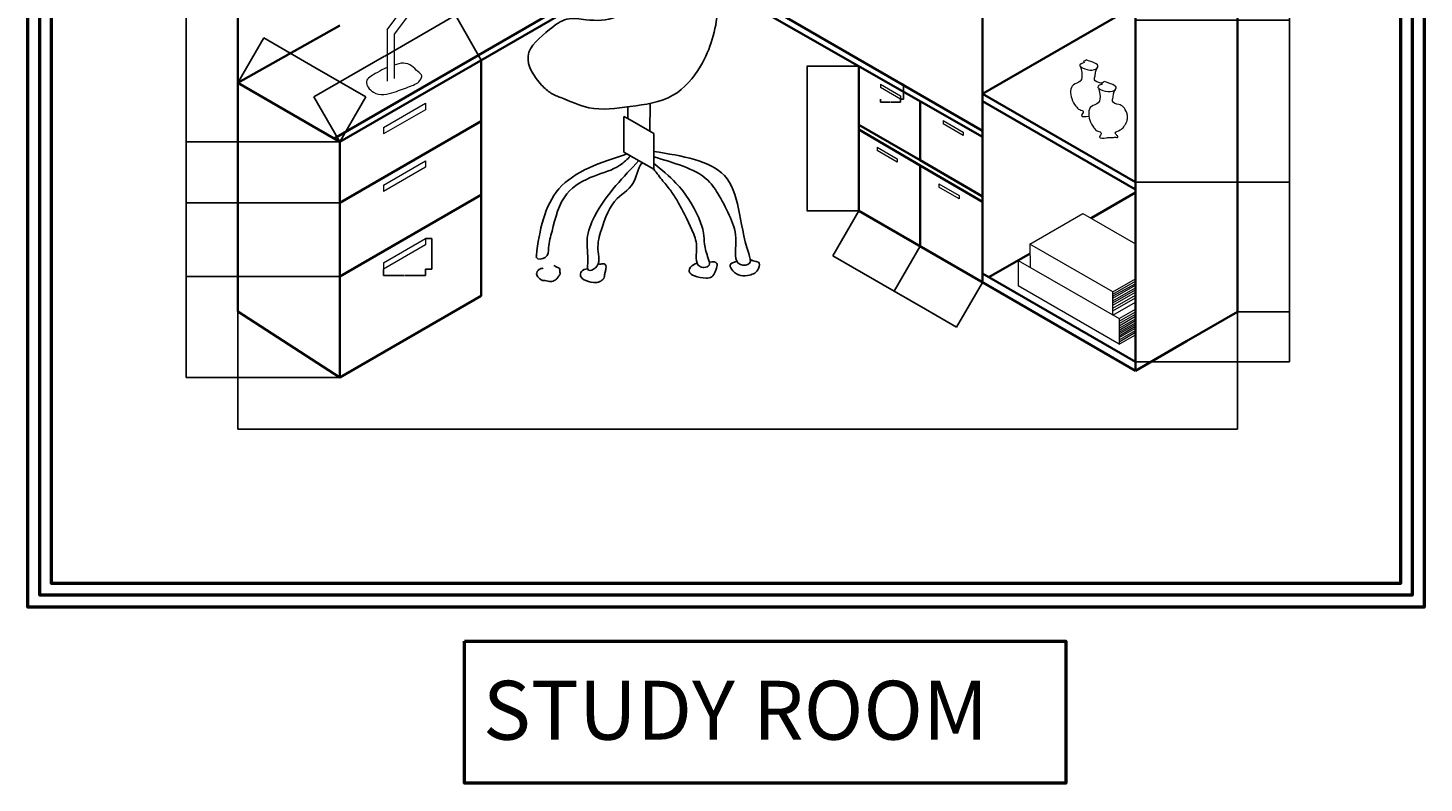
# Model space of a CAD drawing. Units: millimetres. Extents: x -2976 to 8877, y -7187 to 5690.
# Tile 1 of 2: x -2976 to 8877, y -7187 to -776. Entities that reach past the tile are written whole.
import ezdxf

# ---------------------------------------------------------------- set-up
doc = ezdxf.new("R2010")
doc.units = ezdxf.units.MM
doc.header["$MEASUREMENT"] = 0
for name, color, linetype, lineweight in [('A-ANNO-DIMS', 2, 'Continuous', 18), ('A-ANNO-TEXT', 7, 'Continuous', 25), ('A-ANNO-TTLB', 7, 'Continuous', 50), ('A-FURN', 7, 'Continuous', 35), ('A-FURN-ACCS', 3, 'Continuous', 18), ('A-FURN-CHAIR', 4, 'Continuous', 25), ('A-FURN-HDWR', 8, 'Continuous', 18)]:
    doc.layers.add(name, color=color, linetype=linetype, lineweight=lineweight)
doc.styles.get("Standard").update_dxf_attribs({"font": 'arial.ttf'})
doc.dimstyles.get("Standard").update_dxf_attribs({"dimtxt": 0.18, "dimasz": 0.18, "dimexe": 0.18, "dimexo": 0.0625, "dimgap": 0.09, "dimtad": 0, "dimtih": 1, "dimtoh": 1, "dimdec": 0, "dimzin": 0, "dimdsep": 46, "dimtxsty": 'Standard', "dimcen": 0.09, "dimadec": 0, "dimazin": 0, "dimtfac": 1, "dimtdec": 0, "dimtofl": 0, "dimtmove": 0, "dimatfit": 3, "dimfxl": 1, "dimtolj": 1, "dimtzin": 0, "dimarcsym": 0})

# ---------------------------------------------------------------- blocks, each defined once
blk = doc.blocks.new('HANDLE-DRAWER-SMALL')
for p, q in [((0.0001567628432895, 127.2617230564292), (171.3484414772911, 28.33374475136225)), ((0.0001567628432895, 127.2617230564292), (0.0001567628432895, 98.92782070625071)), ((171.3484414772911, -0.0001575988162585), (0.0001567628432895, 98.92782070625049)), ((171.3484414772911, 28.33374475136225), (171.3484414772911, -0.0001575988162585))]:
    blk.add_line(p, q)
blk = doc.blocks.new('HANDLE-DRAWER-LARGE')
for p, q in [((-0.0002251850147701, 53.86751840886313), (355.8206058050919, 259.3007709642777)), ((355.820605805092, 259.3007709642777), (355.820605805092, 205.4328967889142)), ((355.820605805092, 205.4328967889142), (-0.000225185014763, -0.0003557665004337)), ((-0.0002251850147701, 53.86751840886313), (-0.0002251850147701, -0.0003557665004337))]:
    blk.add_line(p, q)
blk = doc.blocks.new('*D5')
at = {"layer": 'A-ANNO-DIMS', "color": 0, "lineweight": -2, "transparency": 16777216}
for p, q in [((4261.184156762843, -1380.200657598816), (4261.184156762843, -1406.020400305983)), ((4261.364156762843, -1405.840400305983), (4344.674786159631, -1405.840400305983)), ((4432.352441477291, -1405.840400305983), (4349.041812080504, -1405.840400305983)), ((4432.532441477291, -1380.200657598816), (4432.532441477291, -1406.020400305983))]:
    blk.add_line(p, q, dxfattribs=at)
at = {"layer": 'A-ANNO-DIMS', "color": 0, "transparency": 16777216}
for points in [[(4261.364156762843, -1405.810400305983), (4261.364156762843, -1405.870400305983), (4261.184156762843, -1405.840400305983)], [(4432.352441477291, -1405.810400305983), (4432.352441477291, -1405.870400305983), (4432.532441477291, -1405.840400305983)]]:
    blk.add_solid(points, dxfattribs=at)
at = {"layer": 'Defpoints', "color": 0, "transparency": 16777216}
for p in [(4261.184156762843, -1380.138157598816), (4432.532441477291, -1380.138157598816), (4432.532441477291, -1405.840400305983)]:
    blk.add_point(p, dxfattribs=at)
at = {"layer": 'A-ANNO-DIMS', "color": 0, "transparency": 16777216, "insert": (4346.858299120067, -1405.840400305983), "char_height": 0.18, "attachment_point": 5}
blk.add_mtext('\\A1;SMALL DRAWER HANDLE 171 TYP.', dxfattribs=at)
blk = doc.blocks.new('*D6')
at = {"layer": 'A-ANNO-DIMS', "color": 0, "lineweight": -2, "transparency": 16777216}
for p, q in [((4432.594941477293, -1252.876276943571), (4458.414684184462, -1252.876276943571)), ((4458.234684184462, -1253.056276943571), (4458.234684184462, -1316.326787530402)), ((4432.594941477293, -1380.138157598816), (4458.414684184462, -1380.138157598816)), ((4458.234684184462, -1379.958157598816), (4458.234684184462, -1316.687647011985))]:
    blk.add_line(p, q, dxfattribs=at)
at = {"layer": 'A-ANNO-DIMS', "color": 0, "transparency": 16777216}
for points in [[(4458.204684184462, -1253.056276943571), (4458.264684184461, -1253.056276943571), (4458.234684184462, -1252.876276943571)], [(4458.204684184462, -1379.958157598816), (4458.264684184461, -1379.958157598816), (4458.234684184462, -1380.138157598816)]]:
    blk.add_solid(points, dxfattribs=at)
at = {"layer": 'Defpoints', "color": 0, "transparency": 16777216}
for p in [(4432.532441477293, -1252.876276943571), (4458.234684184462, -1252.876276943571), (4432.532441477293, -1380.138157598816)]:
    blk.add_point(p, dxfattribs=at)
at = {"layer": 'A-ANNO-DIMS', "color": 0, "transparency": 16777216, "insert": (4458.234684184461, -1316.507217271195), "char_height": 0.18, "attachment_point": 5}
blk.add_mtext('\\A1;127 TYP.', dxfattribs=at)
blk = doc.blocks.new('*D7')
at = {"layer": 'A-ANNO-DIMS', "color": 0, "lineweight": -2, "transparency": 16777216}
for p, q in [((42.54377481498502, -2823.755194985225), (42.54377481498502, -2877.245819633741)), ((398.3646058050918, -2823.755194985225), (398.3646058050918, -2877.245819633741)), ((42.72377481498502, -2877.06581963374), (218.2603021790698, -2877.06581963374)), ((398.1846058050918, -2877.06581963374), (222.648078441007, -2877.06581963374))]:
    blk.add_line(p, q, dxfattribs=at)
at = {"layer": 'A-ANNO-DIMS', "color": 0, "transparency": 16777216}
for points in [[(42.72377481498502, -2877.03581963374), (42.72377481498502, -2877.095819633741), (42.54377481498502, -2877.06581963374)], [(398.1846058050918, -2877.03581963374), (398.1846058050918, -2877.095819633741), (398.3646058050918, -2877.06581963374)]]:
    blk.add_solid(points, dxfattribs=at)
at = {"layer": 'Defpoints', "color": 0, "transparency": 16777216}
for p in [(42.54377481498502, -2823.692694985225), (398.3646058050918, -2823.692694985225), (398.3646058050918, -2877.06581963374)]:
    blk.add_point(p, dxfattribs=at)
at = {"layer": 'A-ANNO-DIMS', "color": 0, "transparency": 16777216, "insert": (220.4541903100384, -2877.06581963374), "char_height": 0.18, "attachment_point": 5}
blk.add_mtext('\\A1;LARGE DRAWER HANDLE 356 TYP.', dxfattribs=at)
blk = doc.blocks.new('*D8')
at = {"layer": 'A-ANNO-DIMS', "color": 0, "lineweight": -2, "transparency": 16777216}
for p, q in [((398.427105805092, -2564.391568254448), (451.9177304536082, -2564.391568254448)), ((451.7377304536082, -2564.571568254447), (451.7377304536082, -2693.860228482047)), ((451.7377304536082, -2823.512694985226), (451.7377304536082, -2694.224034757627)), ((398.427105805092, -2823.692694985226), (451.9177304536082, -2823.692694985226))]:
    blk.add_line(p, q, dxfattribs=at)
at = {"layer": 'A-ANNO-DIMS', "color": 0, "transparency": 16777216}
for points in [[(451.7077304536082, -2564.571568254447), (451.7677304536081, -2564.571568254447), (451.7377304536082, -2564.391568254448)], [(451.7077304536083, -2823.512694985226), (451.7677304536082, -2823.512694985226), (451.7377304536082, -2823.692694985226)]]:
    blk.add_solid(points, dxfattribs=at)
at = {"layer": 'Defpoints', "color": 0, "transparency": 16777216}
for p in [(398.364605805092, -2564.391568254448), (451.7377304536082, -2564.391568254448), (398.364605805092, -2823.692694985226)]:
    blk.add_point(p, dxfattribs=at)
at = {"layer": 'A-ANNO-DIMS', "color": 0, "transparency": 16777216, "insert": (451.7377304536073, -2694.042131619836), "char_height": 0.18, "attachment_point": 5}
blk.add_mtext('\\A1;259 TYP.', dxfattribs=at)
blk = doc.blocks.new('*D13')
at = {"layer": 'A-ANNO-DIMS', "color": 0, "lineweight": -2, "transparency": 16777216}
for p, q in [((-1193.667478, -3183.97615), (-1193.667478, -4182.681808)), ((7293.381479, -3185.702519), (7293.381479, -4182.681808)), ((-1193.487478, -4182.501808), (3049.498105547749, -4182.501808)), ((7293.201479, -4182.501808), (3050.215895452251, -4182.501808))]:
    blk.add_line(p, q, dxfattribs=at)
at = {"layer": 'A-ANNO-DIMS', "color": 0, "transparency": 16777216}
for points in [[(-1193.487478, -4182.471808), (-1193.487478, -4182.531807999999), (-1193.667478, -4182.501808)], [(7293.201479, -4182.471808), (7293.201479, -4182.531807999999), (7293.381479, -4182.501808)]]:
    blk.add_solid(points, dxfattribs=at)
at = {"layer": 'Defpoints', "color": 0, "transparency": 16777216}
for p in [(-1193.667478, -3183.91365), (7293.381479, -3185.640019), (7293.381479, -4182.501808)]:
    blk.add_point(p, dxfattribs=at)
at = {"layer": 'A-ANNO-DIMS', "color": 0, "transparency": 16777216, "insert": (3049.8570005, -4182.501808), "char_height": 0.18, "attachment_point": 5}
blk.add_mtext('\\A1;8487', dxfattribs=at)
blk = doc.blocks.new('*D14')
at = {"layer": 'A-ANNO-DIMS', "color": 0, "lineweight": -2, "transparency": 16777216}
for p, q in [((2530.179259000001, 4564.359981000001), (-1633.847478000003, 4564.359981)), ((-1633.667478000003, 4564.179981), (-1633.667478000002, 411.1110510293304)), ((-1633.667478000001, -3742.321808000003), (-1633.667478000002, 410.7471219706673)), ((-327.7045740000001, -3742.501808000002), (-1633.847478000001, -3742.501808000002))]:
    blk.add_line(p, q, dxfattribs=at)
at = {"layer": 'A-ANNO-DIMS', "color": 0, "transparency": 16777216}
for points in [[(-1633.697478000003, 4564.179981), (-1633.637478000003, 4564.179981), (-1633.667478000003, 4564.359981)], [(-1633.697478000001, -3742.321808000003), (-1633.637478000001, -3742.321808000003), (-1633.667478000001, -3742.501808000002)]]:
    blk.add_solid(points, dxfattribs=at)
at = {"layer": 'Defpoints', "color": 0, "transparency": 16777216}
for p in [(2530.241759000001, 4564.359981000001), (-1633.667478000001, -3742.501808000002), (-327.6420740000001, -3742.501808000002)]:
    blk.add_point(p, dxfattribs=at)
at = {"layer": 'A-ANNO-DIMS', "color": 0, "transparency": 16777216, "insert": (-1633.667478000001, 410.9290864999992), "char_height": 0.18, "attachment_point": 5}
blk.add_mtext('\\A1;8307', dxfattribs=at)
blk = doc.blocks.new('*D15')
at = {"layer": 'A-ANNO-DIMS', "color": 0, "lineweight": -2, "transparency": 16777216}
for p, q in [((7293.443979000004, 1814.359981000001), (7733.561479000008, 1814.359981000001)), ((7733.381479000008, 1814.179981000001), (7733.381479000008, -685.4581158622104)), ((7733.381479000008, -3185.460019000002), (7733.381479000008, -685.8219221377904)), ((7293.443979000004, -3185.640019000002), (7733.561479000008, -3185.640019000002))]:
    blk.add_line(p, q, dxfattribs=at)
at = {"layer": 'A-ANNO-DIMS', "color": 0, "transparency": 16777216}
for points in [[(7733.351479000008, 1814.179981000001), (7733.411479000007, 1814.179981000001), (7733.381479000008, 1814.359981000001)], [(7733.351479000008, -3185.460019000002), (7733.411479000007, -3185.460019000002), (7733.381479000008, -3185.640019000002)]]:
    blk.add_solid(points, dxfattribs=at)
at = {"layer": 'Defpoints', "color": 0, "transparency": 16777216}
for p in [(7293.381479000003, 1814.359981000001), (7293.381479000003, -3185.640019000002), (7733.381479000008, -3185.640019000002)]:
    blk.add_point(p, dxfattribs=at)
at = {"layer": 'A-ANNO-DIMS', "color": 0, "transparency": 16777216, "insert": (7733.381479000005, -685.6400190000024), "char_height": 0.18, "attachment_point": 5}
blk.add_mtext('\\A1;5000', dxfattribs=at)
blk = doc.blocks.new('*D20')
at = {"layer": 'A-ANNO-DIMS', "color": 0, "lineweight": -2, "transparency": 16777216}
for p, q in [((-327.7045740000001, -1742.087738000001), (-1633.847478000002, -1742.087738000001)), ((-1633.667478000002, -1742.267738000001), (-1633.667478000002, -2000.780451862212)), ((-1633.667478000002, -2259.656972000001), (-1633.667478000002, -2001.144258137792)), ((-327.7045740000001, -2259.836972000001), (-1633.847478000002, -2259.836972000002))]:
    blk.add_line(p, q, dxfattribs=at)
at = {"layer": 'A-ANNO-DIMS', "color": 0, "transparency": 16777216}
for points in [[(-1633.697478000002, -1742.267738000001), (-1633.637478000002, -1742.267738000001), (-1633.667478000002, -1742.087738000001)], [(-1633.697478000002, -2259.656972000001), (-1633.637478000002, -2259.656972000001), (-1633.667478000002, -2259.836972000002)]]:
    blk.add_solid(points, dxfattribs=at)
at = {"layer": 'Defpoints', "color": 0, "transparency": 16777216}
for p in [(-327.6420740000001, -1742.087738000001), (-1633.667478000002, -2259.836972000002), (-327.6420740000001, -2259.836972000001)]:
    blk.add_point(p, dxfattribs=at)
at = {"layer": 'A-ANNO-DIMS', "color": 0, "transparency": 16777216, "insert": (-1633.667478000002, -2000.962355000001), "char_height": 0.18, "attachment_point": 5}
blk.add_mtext('\\A1;517.7', dxfattribs=at)
blk = doc.blocks.new('*D21')
at = {"layer": 'A-ANNO-DIMS', "color": 0, "lineweight": -2, "transparency": 16777216}
for p, q in [((-327.7045740000001, -2259.836972000001), (-1633.847478000002, -2259.836972000002)), ((-1633.667478000002, -2260.016972000002), (-1633.667478000002, -2572.29027447067)), ((-1633.667478000002, -2884.927506000002), (-1633.667478000002, -2572.654203529334)), ((-327.7045740000001, -2885.107506000001), (-1633.847478000001, -2885.107506000002))]:
    blk.add_line(p, q, dxfattribs=at)
at = {"layer": 'A-ANNO-DIMS', "color": 0, "transparency": 16777216}
for points in [[(-1633.697478000002, -2260.016972000002), (-1633.637478000002, -2260.016972000002), (-1633.667478000002, -2259.836972000002)], [(-1633.697478000002, -2884.927506000002), (-1633.637478000002, -2884.927506000002), (-1633.667478000002, -2885.107506000002)]]:
    blk.add_solid(points, dxfattribs=at)
at = {"layer": 'Defpoints', "color": 0, "transparency": 16777216}
for p in [(-327.6420740000001, -2259.836972000001), (-1633.667478000002, -2885.107506000002), (-327.6420740000001, -2885.107506000001)]:
    blk.add_point(p, dxfattribs=at)
at = {"layer": 'A-ANNO-DIMS', "color": 0, "transparency": 16777216, "insert": (-1633.667478000002, -2572.472239000001), "char_height": 0.18, "attachment_point": 5}
blk.add_mtext('\\A1;625.3', dxfattribs=at)
blk = doc.blocks.new('*D22')
at = {"layer": 'A-ANNO-DIMS', "color": 0, "lineweight": -2, "transparency": 16777216}
for p, q in [((-327.7045740000001, -2885.107506000001), (-1633.847478000001, -2885.107506000002)), ((-1633.667478000002, -2885.287506000001), (-1633.667478000002, -3313.622753862212)), ((-1633.667478000002, -3742.321808000003), (-1633.667478000002, -3313.986560137792)), ((-327.7045740000001, -3742.501808000002), (-1633.847478000002, -3742.501808000002))]:
    blk.add_line(p, q, dxfattribs=at)
at = {"layer": 'A-ANNO-DIMS', "color": 0, "transparency": 16777216}
for points in [[(-1633.697478000002, -2885.287506000001), (-1633.637478000002, -2885.287506000001), (-1633.667478000002, -2885.107506000002)], [(-1633.697478000001, -3742.321808000003), (-1633.637478000002, -3742.321808000003), (-1633.667478000002, -3742.501808000002)]]:
    blk.add_solid(points, dxfattribs=at)
at = {"layer": 'Defpoints', "color": 0, "transparency": 16777216}
for p in [(-327.6420740000001, -2885.107506000001), (-1633.667478000002, -3742.501808000002), (-327.6420740000001, -3742.501808000002)]:
    blk.add_point(p, dxfattribs=at)
at = {"layer": 'A-ANNO-DIMS', "color": 0, "transparency": 16777216, "insert": (-1633.667478000002, -3313.804657000001), "char_height": 0.18, "attachment_point": 5}
blk.add_mtext('\\A1;857.4', dxfattribs=at)
blk = doc.blocks.new('*D23')
at = {"layer": 'A-ANNO-DIMS', "color": 0, "lineweight": -2, "transparency": 16777216}
for p, q in [((-1193.636228, -1242.033611412263), (-973.5774778280621, -860.8806754643598)), ((-973.5115932553808, -861.1265600370411), (-540.9698413317153, -1110.854656945921)), ((-107.7979584546333, -1360.946560130381), (-540.3397103782987, -1111.218463221501)), ((-327.6108240000001, -1742.033611412263), (-107.5520738819521, -1360.8806755577))]:
    blk.add_line(p, q, dxfattribs=at)
at = {"layer": 'A-ANNO-DIMS', "color": 0, "transparency": 16777216}
for points in [[(-973.4965932553808, -861.1005792749278), (-973.526593255381, -861.1525407991548), (-973.6674778280621, -861.0365600370412)], [(-107.7829584546333, -1360.920579368268), (-107.8129584546333, -1360.972540892495), (-107.6420738819521, -1361.036560130381)]]:
    blk.add_solid(points, dxfattribs=at)
at = {"layer": 'Defpoints', "color": 0, "transparency": 16777216}
for p in [(-1193.667478, -1242.087738), (-107.6420738819521, -1361.036560130381), (-327.642074, -1742.087738)]:
    blk.add_point(p, dxfattribs=at)
at = {"layer": 'A-ANNO-DIMS', "color": 0, "transparency": 16777216, "insert": (-540.654775855007, -1111.036560083711), "char_height": 0.18, "attachment_point": 5}
blk.add_mtext('\\A1;1000', dxfattribs=at)
blk = doc.blocks.new('*D24')
at = {"layer": 'A-ANNO-DIMS', "color": 0, "lineweight": -2, "transparency": 16777216}
for p, q in [((652.7837904139722, -667.9703643117301), (52.96397228998472, -1014.276497770886)), ((872.9084249999999, -1048.877415412263), (652.8496749866534, -667.7244797390488)), ((-547.4861894539579, -1360.946560288706), (52.33362867002966, -1014.640426829549)), ((-327.6733239999999, -1742.033611412263), (-547.7320740266391, -1360.880675716025))]:
    blk.add_line(p, q, dxfattribs=at)
at = {"layer": 'A-ANNO-DIMS', "color": 0, "transparency": 16777216}
for points in [[(652.7687904139723, -667.9443835496166), (652.7987904139723, -667.9963450738435), (652.9396749866535, -667.8803643117301)], [(-547.5011894539577, -1360.920579526592), (-547.4711894539579, -1360.972541050819), (-547.6420740266392, -1361.036560288706)]]:
    blk.add_solid(points, dxfattribs=at)
at = {"layer": 'Defpoints', "color": 0, "transparency": 16777216}
for p in [(652.9396749866535, -667.8803643117301), (872.9396749999999, -1048.931542), (-327.6420739999999, -1742.087737999999)]:
    blk.add_point(p, dxfattribs=at)
at = {"layer": 'A-ANNO-DIMS', "color": 0, "transparency": 16777216, "insert": (52.64880048000714, -1014.458462300218), "char_height": 0.18, "attachment_point": 5}
blk.add_mtext('\\A1;1386.3', dxfattribs=at)
blk = doc.blocks.new('*D37')
at = {"layer": 'A-ANNO-DIMS', "color": 0, "lineweight": -2, "transparency": 16777216}
for p, q in [((6427.418576000004, -709.7861090000002), (7733.561479000008, -709.7861090000001)), ((7733.381479000008, -709.966109), (7733.381479000008, -1397.385788970669)), ((7733.381479000008, -2085.169398000001), (7733.381479000008, -1397.749718029332)), ((6427.418576000004, -2085.349398000001), (7733.561479000008, -2085.349398))]:
    blk.add_line(p, q, dxfattribs=at)
at = {"layer": 'A-ANNO-DIMS', "color": 0, "transparency": 16777216}
for points in [[(7733.351479000008, -709.966109), (7733.411479000007, -709.966109), (7733.381479000008, -709.7861090000001)], [(7733.351479000008, -2085.169398000001), (7733.411479000007, -2085.169398000001), (7733.381479000008, -2085.349398)]]:
    blk.add_solid(points, dxfattribs=at)
at = {"layer": 'Defpoints', "color": 0, "transparency": 16777216}
for p in [(6427.356076000004, -709.7861090000002), (6427.356076000004, -2085.349398000001), (7733.381479000008, -2085.349398)]:
    blk.add_point(p, dxfattribs=at)
at = {"layer": 'A-ANNO-DIMS', "color": 0, "transparency": 16777216, "insert": (7733.381479000005, -1397.567753500002), "char_height": 0.18, "attachment_point": 5}
blk.add_mtext('\\A1;1375.6', dxfattribs=at)
blk = doc.blocks.new('*D38')
at = {"layer": 'A-ANNO-DIMS', "color": 0, "lineweight": -2, "transparency": 16777216}
for p, q in [((6427.418576000004, -2085.349398000001), (7733.561479000008, -2085.349398)), ((7733.381479000008, -2085.529398), (7733.381479000008, -2848.216410862211)), ((7733.381479000008, -3611.267230000002), (7733.381479000008, -2848.58021713779)), ((6427.418576000004, -3611.447230000003), (7733.561479000008, -3611.447230000002))]:
    blk.add_line(p, q, dxfattribs=at)
at = {"layer": 'A-ANNO-DIMS', "color": 0, "transparency": 16777216}
for points in [[(7733.351479000008, -2085.529398), (7733.411479000007, -2085.529398), (7733.381479000008, -2085.349398)], [(7733.351479000008, -3611.267230000002), (7733.411479000007, -3611.267230000002), (7733.381479000008, -3611.447230000002)]]:
    blk.add_solid(points, dxfattribs=at)
at = {"layer": 'Defpoints', "color": 0, "transparency": 16777216}
for p in [(6427.356076000004, -2085.349398000001), (6427.356076000004, -3611.447230000003), (7733.381479000008, -3611.447230000002)]:
    blk.add_point(p, dxfattribs=at)
at = {"layer": 'A-ANNO-DIMS', "color": 0, "transparency": 16777216, "insert": (7733.381479000005, -2848.398314000002), "char_height": 0.18, "attachment_point": 5}
blk.add_mtext('\\A1;1526', dxfattribs=at)
blk = doc.blocks.new('*D39')
at = {"layer": 'A-ANNO-DIMS', "color": 0, "lineweight": -2, "transparency": 16777216}
for p, q in [((4078.281165000002, -1100.041375), (3638.163665000004, -1100.041375)), ((3638.343665000004, -1100.221375), (3638.343665000004, -1714.557320362211)), ((3638.343665000004, -2329.257072000001), (3638.343665000004, -1714.921126637791)), ((4078.281165000002, -2329.437072000001), (3638.163665000004, -2329.437072000001))]:
    blk.add_line(p, q, dxfattribs=at)
at = {"layer": 'A-ANNO-DIMS', "color": 0, "transparency": 16777216}
for points in [[(3638.313665000004, -1100.221375), (3638.373665000004, -1100.221375), (3638.343665000004, -1100.041375)], [(3638.313665000004, -2329.257072000001), (3638.373665000004, -2329.257072000001), (3638.343665000004, -2329.437072000001)]]:
    blk.add_solid(points, dxfattribs=at)
at = {"layer": 'Defpoints', "color": 0, "transparency": 16777216}
for p in [(3638.343665000004, -1100.041375), (4078.343665000002, -1100.041375), (4078.343665000002, -2329.437072000001)]:
    blk.add_point(p, dxfattribs=at)
at = {"layer": 'A-ANNO-DIMS', "color": 0, "transparency": 16777216, "insert": (3638.343665000002, -1714.739223500002), "char_height": 0.18, "attachment_point": 5}
blk.add_mtext('\\A1;1229.4', dxfattribs=at)
blk = doc.blocks.new('*D40')
at = {"layer": 'A-ANNO-DIMS', "color": 0, "lineweight": -2, "transparency": 16777216}
for p, q in [((4078.312415, -2329.491198587737), (3858.25366514816, -2710.644133981217)), ((3858.499549720842, -2710.578249408535), (4117.930722219806, -2860.360906686992)), ((4598.116659999999, -2629.600319587737), (4378.057910244868, -3010.75325481371)), ((4377.992025672187, -3010.507370241029), (4118.560853173222, -2860.724712962572))]:
    blk.add_line(p, q, dxfattribs=at)
at = {"layer": 'A-ANNO-DIMS', "color": 0, "transparency": 16777216}
for points in [[(3858.514549720842, -2710.552268646422), (3858.484549720842, -2710.604230170649), (3858.343665148161, -2710.488249408535)], [(4378.007025672188, -3010.481389478915), (4377.977025672186, -3010.533351003143), (4378.147910244869, -3010.597370241029)]]:
    blk.add_solid(points, dxfattribs=at)
at = {"layer": 'Defpoints', "color": 0, "transparency": 16777216}
for p in [(4078.343665000001, -2329.437072000001), (3858.343665148161, -2710.488249408535), (4598.147909999999, -2629.546193)]:
    blk.add_point(p, dxfattribs=at)
at = {"layer": 'A-ANNO-DIMS', "color": 0, "transparency": 16777216, "insert": (4118.245787696515, -2860.542809824782), "char_height": 0.18, "attachment_point": 5}
blk.add_mtext('\\A1;600.2', dxfattribs=at)
blk = doc.blocks.new('*D41')
at = {"layer": 'A-ANNO-DIMS', "color": 0, "lineweight": -2, "transparency": 16777216}
for p, q in [((4598.116659999999, -2629.600319587737), (4378.057910040612, -3010.75325516749)), ((5128.286719999999, -2935.694145587736), (4908.2279696694, -3316.84708181045)), ((4378.303794613294, -3010.687370594808), (4642.917874378298, -3163.462380778498)), ((4908.162085096718, -3316.601197237768), (4643.548005331715, -3163.826187054079))]:
    blk.add_line(p, q, dxfattribs=at)
at = {"layer": 'A-ANNO-DIMS', "color": 0, "transparency": 16777216}
for points in [[(4378.318794613295, -3010.661389832695), (4378.288794613294, -3010.713351356922), (4378.147910040612, -3010.597370594808)], [(4908.177085096719, -3316.575216475654), (4908.147085096718, -3316.627177999882), (4908.3179696694, -3316.691197237768)]]:
    blk.add_solid(points, dxfattribs=at)
at = {"layer": 'Defpoints', "color": 0, "transparency": 16777216}
for p in [(4598.147909999999, -2629.546193), (5128.317969999999, -2935.640019), (4378.147910040612, -3010.597370594808)]:
    blk.add_point(p, dxfattribs=at)
at = {"layer": 'A-ANNO-DIMS', "color": 0, "transparency": 16777216, "insert": (4643.232939855005, -3163.644283916288), "char_height": 0.18, "attachment_point": 5}
blk.add_mtext('\\A1;612.2', dxfattribs=at)

msp = doc.modelspace()

# ---------------------------------------------------------------- linework, layer by layer
at = {"layer": 'A-ANNO-TTLB'}
for points in [[(-2976.020185178524, 5689.883775799608), (8877.112005194242, 5689.883775799608), (8877.112005194242, -5692.972772104557), (-2976.020185178524, -5692.972772104557)], [(-2876.020185178524, 5589.883775799608), (8777.112005194242, 5589.883775799608), (8777.112005194242, -5592.972772104559), (-2876.020185178524, -5592.972772104556)], [(-2776.020185178524, 5489.883775799608), (8677.112005194242, 5489.883775799608), (8677.112005194242, -5492.972772104557), (-2776.020185178524, -5492.972772104557)], [(730.558269318426, -5982.695910667484), (5834.908152036602, -5982.695910667484), (5834.908152036602, -7187.111297581913), (730.558269318426, -7187.111297581913)]]:
    msp.add_lwpolyline(points, close=True, dxfattribs=at)
at = {"layer": 'A-FURN'}
for p, q in [((5128.317970011113, 2064.359980599719), (5128.317970011111, -2935.640019400281)), ((7293.381479472209, -3185.640019400281), (7293.381479472209, 1814.35998059972)), ((6427.35607568777, -1085.64001940028), (6427.35607568777, 1314.359980599719)), ((-1193.66747761529, -254.7515361428099), (-1193.66747761529, -1242.087737987627)), ((-376.8059096461261, -1713.702984145284), (2154.739901078788, -252.1143288573858)), ((-327.6420738308511, -1742.087737987627), (2160.78160776331, -305.3956555613991)), ((5128.317970011111, -1648.386495488528), (2868.673209343396, -343.7799846440953)), ((2876.002629457045, -413.7919664145265), (5128.31797001111, -1699.325791095172)), ((5128.317970011111, -1335.349397541315), (6275.967791248173, -672.7534643146713)), ((-1193.66747761529, -1242.087737987628), (-327.642073830851, -754.7515361428099)), ((872.9396751026754, -1048.931542056704), (872.9396751026754, -3049.345612309716)), ((4078.343665064641, -1100.04137485433), (4078.343665064641, -2329.437071797247)), ((6427.35607568777, -1285.64001940028), (6427.35607568777, -1085.64001940028)), ((-327.6420738308511, -1742.087737987627), (-1193.66747761529, -1242.087737987628)), ((-1193.66747761529, -1242.087737987627), (-1193.66747761529, -3183.913650243725)), ((6427.35607568777, -3685.640019400282), (6427.35607568777, -1285.64001940028)), ((4598.147910479227, -1899.687531258836), (4598.147910479227, -1396.725381601212)), ((5128.317970011111, -1335.349397541315), (6427.35607568777, -2085.349397541316)), ((5128.317970011113, -1398.749974361068), (6427.356075687772, -2148.749974361068)), ((-327.6420738308511, -2259.836972325146), (872.9396751026754, -1566.680776394222)), ((4078.343665064641, -1638.419219015341), (4078.343665064641, -1580.825336966307)), ((4598.147910479227, -1899.687531258836), (4078.343665064641, -1599.578410242815)), ((4598.147910479227, -1944.215401092574), (4078.343665064641, -1638.419219015341)), ((-327.6420738308511, -1742.087737987627), (-327.6420738308511, -3742.501808240639)), ((4598.147910479227, -1899.687531258836), (5128.31797001111, -2206.130517844991)), ((4598.147910479227, -2629.546192813267), (4598.147910479227, -1944.215401092574)), ((5128.31797001111, -2251.382858366319), (4598.147910479227, -1944.215401092574)), ((872.9396751026754, -2191.951310376734), (-327.6420738308511, -2885.107506307658)), ((5128.31797001111, -2206.130517844991), (5128.31797001111, -2251.382858366319)), ((6050.637307758741, -2391.169290330906), (6427.35607568777, -2173.670608258297)), ((5117.952155893814, -2929.655313829289), (4078.343665064641, -2329.437071797246)), ((5182.204996154414, -2892.558919208634), (5531.727093629879, -2690.762242143452)), ((5117.952155893814, -2929.655313829289), (5128.317970011111, -2923.670608258298)), ((6427.35607568777, -3685.64001940028), (5117.952155893814, -2929.655313829289)), ((5128.317970011111, -2861.447230158971), (6427.356075687768, -3611.44723015897)), ((-327.6420738308511, -3742.501808240639), (872.9396751026754, -3049.345612309716)), ((-1193.66747761529, -3183.913650243725), (-327.6420738308511, -3742.501808240639)), ((6860.368777579989, -3435.64001940028), (7293.381479472209, -3185.640019400281)), ((6427.35607568777, -3685.64001940028), (6860.368777579989, -3435.64001940028))]:
    msp.add_line(p, q, dxfattribs=at)
at = {"layer": 'A-FURN-ACCS'}
for p, q in [((74.7991430560337, -791.1457519195437), (702.1545995256746, 63.22767765958269)), ((720.8745203412259, -47.45045240482432), (132.6519606441791, -828.0224899209036)), ((74.7991430560337, -791.1457519195433), (74.7991430560337, -1228.692969014349)), ((132.6519606441789, -828.0224899209036), (132.6519606441789, -1203.815902757262)), ((5531.269034738128, -2610.703217742857), (5981.075129379752, -2351.007547918381)), ((5981.075129379752, -2351.007547918381), (6427.35607568777, -2608.667972403516)), ((5430.850081920362, -2749.003612008986), (5531.727093629879, -2690.762242143452)), ((6235.446123861315, -3017.260049705295), (5531.269034738128, -2610.703217742857)), ((5531.269034738128, -2610.703217742857), (5532.395760165672, -2807.631036678959)), ((5430.850081920362, -2749.003612008986), (6287.514215480928, -3243.598880125276)), ((5430.850081920362, -2749.003612008986), (5430.850081920361, -2966.269631675821)), ((6235.446123861315, -3017.260049705295), (6427.35607568777, -2906.460787358123)), ((6235.446123861315, -3035.176497082961), (6425.910328665804, -2925.2119371681)), ((6427.35607568777, -2947.92894271249), (6235.446123861315, -3051.832811871252)), ((6235.446123861315, -3070.075531782983), (6427.35607568777, -2959.276269435811)), ((6425.910328665804, -2925.2119371681), (6427.35607568777, -2947.92894271249)), ((6287.514215480928, -3460.864899792112), (5430.850081920362, -2966.269631675821)), ((6235.446123861315, -3092.790260193877), (6427.35607568777, -2981.990997846704)), ((6235.446123861315, -3110.483757676251), (6427.35607568777, -2999.684495329079)), ((6235.446123861315, -3213.537353412503), (6235.446123861315, -3017.260049705295)), ((6235.446123861315, -3129.72940268684), (6427.35607568777, -3018.930140339669)), ((6235.446123861315, -3154.252012545709), (6427.35607568777, -3043.452750198537)), ((6235.446123861315, -3051.832811871252), (6235.446123861315, -3070.075531782983)), ((6235.446123861315, -3178.869883127795), (6427.35607568777, -3068.070620780622)), ((6235.446123861315, -3213.537353412503), (6427.35607568777, -3102.738091065331)), ((6287.514215480928, -3243.598880125276), (6427.35607568777, -3162.861144490878)), ((6287.514215480928, -3265.620151914605), (6427.35607568777, -3184.882416280207)), ((6287.514215480928, -3285.860691888308), (6427.35607568777, -3205.122956253909)), ((6287.514215480928, -3303.864644779984), (6427.35607568777, -3223.126909145584)), ((6287.514215480928, -3243.598880125276), (6287.514215480928, -3460.864899792112)), ((6287.514215480928, -3325.283153859913), (6427.35607568777, -3244.545418225513)), ((6287.514215480928, -3340.803787272947), (6427.35607568777, -3260.06605163855)), ((6287.514215480928, -3360.049432283537), (6427.35607568777, -3279.311696649137)), ((6287.514215480928, -3373.086746217917), (6427.35607568777, -3292.349010583517)), ((6287.514215480928, -3389.301662576953), (6427.35607568777, -3308.563926942554)), ((6287.514215480928, -3404.822360749146), (6427.35607568777, -3324.084625114747)), ((6287.514215480928, -3424.999177710168), (6427.35607568777, -3344.261442075769)), ((6287.514215480928, -3439.899029822912), (6427.35607568777, -3359.161294188513)), ((6287.514215480928, -3460.864899792112), (6427.35607568777, -3380.127164157713))]:
    msp.add_line(p, q, dxfattribs=at)
for points, knots in [([(6008.317838193092, -1047.783695894715), (6062.007278344803, -1064.373011076868), (6141.676364538607, -1088.989687604105), (6052.297700542336, -1157.616844043003), (5900.862294362656, -1090.215132796341), (6001.792843024243, -1069.431145026291), (5978.712876415237, -1061.328095514574), (5994.661629571309, -1057.404850627941), (6000.613430234271, -1053.425769953793), (6004.95388119505, -1051.516105323734), (6007.267639226588, -1048.948922598626), (6008.317838193092, -1047.783695894715)], [0, 0, 0, 0, 115.4373651336158, 171.2960568563994, 279.0731841669098, 306.4387679226323, 312.7692218456463, 327.1537514953741, 330.4307730061897, 336.0614474905891, 340.7413462684733, 340.7413462684733, 340.7413462684733, 340.7413462684733]), ([(47.52410865535193, -1122.464477650352), (23.87370988971571, -1135.637050931516), (-27.46818392898365, -1164.232968718035), (-136.2274615603337, -1224.504726851633), (-26.40520048521478, -1365.339658644356), (129.510627151118, -1324.292142162895), (256.7858450652411, -1276.704323693345), (351.8440151129968, -1239.762451039769), (374.7245567037771, -1174.08066151128), (324.9854100483347, -1141.005161303983), (285.5270422639212, -1094.812993373568), (208.6564259677015, -1064.214262332315), (158.902898245901, -1082.681696953436), (132.6519606441788, -1092.888711538509)], [0, 0, 0, 0, 85.42412760483053, 185.4445048687641, 293.3346385799873, 470.6804269653958, 617.6169353071942, 722.9136598684736, 753.0724393269832, 801.2529836699167, 873.7077618977403, 945.835179023305, 1028.292071834677, 1028.292071834677, 1028.292071834677, 1028.292071834677]), ([(5958.541580296844, -1102.280952859131), (5963.490180395596, -1119.004156614873), (5975.263600417179, -1158.791025222909), (5973.511460155473, -1238.463478238237), (5868.76945244337, -1252.792841527438), (5873.870399977255, -1368.587848187547), (5913.841085452669, -1434.293974622374), (5945.652475285883, -1471.125174642451), (6000.069181117946, -1479.868932590904), (5942.255690070546, -1536.972764295645), (6005.333678568416, -1528.008568196276), (6029.988515778522, -1525.143977181854), (6031.042003831876, -1525.023859314152)], [0, 0, 0, 0, 53.89871295787923, 128.2326665344357, 194.6274369626239, 311.0043774434725, 386.3724247320341, 430.2818943451568, 463.101306931476, 501.2731315190478, 561.6183083840479, 564.3786332018483, 564.3786332018483, 564.3786332018483, 564.3786332018483]), ([(6137.879473657204, -1245.316562115622), (6135.848210747634, -1244.695004492335), (6112.373641007649, -1237.868369766744), (6067.64457850803, -1228.469876714675), (6086.829368598862, -1179.359431490588), (6086.703059343363, -1143.585952457365), (6099.644910022992, -1121.389754820916), (6105.962418629465, -1110.554776650445)], [1013.087477941611, 1013.087477941611, 1013.087477941611, 1013.087477941611, 1018.898613637143, 1078.679283416861, 1113.127763885908, 1151.570490271903, 1188.232584728662, 1188.232584728662, 1188.232584728662, 1188.232584728662]), ([(6111.842905905994, -1285.327832371003), (6116.791506004748, -1302.051036126745), (6128.564926026329, -1341.837904734782), (6126.812785764625, -1421.510357750109), (6022.070778052519, -1435.839721039311), (6027.171725586406, -1551.634727699418), (6067.142411061821, -1617.340854134246), (6098.953800895034, -1654.172054154323), (6153.370506727096, -1662.915812102777), (6095.557015679696, -1720.019643807517), (6177.718103504886, -1708.343493052847), (6210.806148685501, -1705.432216706824), (6237.969449407291, -1706.485332384098), (6256.70879719548, -1701.904837425191), (6271.855718709359, -1708.556643847699), (6280.245036754393, -1696.232859147447), (6266.266527227525, -1685.181632703388), (6240.675356007846, -1659.705424157168), (6299.912696129545, -1645.638147868136), (6325.87908450043, -1621.655334469943), (6337.008226708871, -1596.707854155097), (6352.237217698235, -1579.994536833868), (6357.250430840323, -1558.609877000696), (6359.226521748699, -1532.268517770606), (6358.616293655167, -1501.548135043027), (6341.580707369659, -1472.688510489718), (6323.253464604221, -1439.036268833873), (6282.132622480866, -1424.373340185241), (6220.945904117183, -1411.516756226548), (6240.130694208012, -1362.40631100246), (6240.004384952515, -1326.632831969237), (6252.946235632141, -1304.436634332789), (6259.263744238616, -1293.601656162317)], [0, 0, 0, 0, 53.89871295787923, 128.2326665344357, 194.6274369626239, 311.0043774434725, 386.3724247320341, 430.2818943451568, 463.101306931476, 501.2731315190478, 561.6183083840479, 595.0182481110646, 620.3011744944619, 639.457999723088, 653.6509631414006, 661.6430805440533, 674.3553248466898, 699.0572658528314, 749.3411743416673, 788.6813671985493, 813.4254089212131, 828.7808019033675, 855.8036652260705, 876.5297583894804, 908.9375671083436, 945.0916138557602, 976.2785553618417, 1018.898613637143, 1078.679283416861, 1113.127763885908, 1151.570490271903, 1188.232584728662, 1188.232584728662, 1188.232584728662, 1188.232584728662]), ([(6161.619163802242, -1230.830575406588), (6215.308603953953, -1247.41989058874), (6294.977690147758, -1272.036567115978), (6205.599026151486, -1340.663723554875), (6054.163619971808, -1273.262012308212), (6155.094168633393, -1252.478024538164), (6132.014202024389, -1244.374975026447), (6147.962955180456, -1240.451730139813), (6153.914755843425, -1236.472649465665), (6158.2552068042, -1234.562984835607), (6160.56896483574, -1231.995802110498), (6161.619163802242, -1230.830575406588)], [0, 0, 0, 0, 115.4373651336158, 171.2960568563994, 279.0731841669098, 306.4387679226323, 312.7692218456463, 327.1537514953741, 330.4307730061897, 336.0614474905891, 340.7413462684733, 340.7413462684733, 340.7413462684733, 340.7413462684733])]:
    msp.add_open_spline(points, degree=3, knots=knots, dxfattribs=at)
msp.add_open_spline([(74.79914305603131, -1113.703174893142), (65.70111388357158, -1116.683431374687), (56.61261126946175, -1119.57395451252), (47.52410865535193, -1122.464477650352)], degree=3, dxfattribs=at)
at = {"layer": 'A-FURN-CHAIR'}
for p, q in [((2303.929857735249, -1653.02189174084), (2306.68403638583, -1416.448466280666)), ((2117.864320687422, -1545.596903839363), (2084.433018706324, -1526.295332641217)), ((2084.433018706324, -1526.295332641217), (2084.433018706324, -1829.563625078688)), ((2117.864320687422, -1446.127502420577), (2117.864320687422, -1545.596903839363)), ((2117.864320687422, -1545.596903839363), (2303.929857735249, -1653.02189174084)), ((2303.929857735249, -1653.02189174084), (2337.414957703552, -1672.35452322138)), ((2337.414957703551, -1672.35452322138), (2337.414957703551, -1975.622815658853)), ((2084.433018706324, -1829.563625078688), (2337.414957703551, -1975.622815658853)), ((2084.433018706324, -1829.563625078688), (2140.652245107687, -1862.021810575148))]:
    msp.add_line(p, q, dxfattribs=at)
for points, knots in [([(2567.327213554687, 217.3777815164612), (2371.604006962237, 192.7327323130228), (2081.31339379434, 156.1799567409558), (2150.139936282865, -182.4667104222866), (2165.116014388808, -365.952377867469), (2201.134482322425, -570.5848202688835), (2001.966179159994, -713.9202466194699), (1796.942794050407, -716.3269363524186), (1590.45379523456, -678.4075351907952), (1425.098437734223, -813.6407202142198), (1195.207760947901, -994.0076673186782), (1334.194099928929, -1211.943894338208), (1433.600624954212, -1310.666009676965), (1490.614413886304, -1345.956672059368), (1614.157571527384, -1391.232703225471), (1813.084480556488, -1488.982700143385), (2144.550172737321, -1441.760630520553), (2511.026644645633, -1393.796613114915), (2787.65137241148, -1067.523731355003), (2900.240674189164, -675.4125804627595), (2869.868896878056, -301.0233351137475), (2802.881672971835, 19.87963263450726), (2647.650590440668, 150.0314944362605), (2567.327213554687, 217.3777815164612)], [0, 0, 0, 0, 465.8253811586821, 690.8978137033012, 888.5150348665003, 1055.970420950123, 1257.901159625074, 1514.322789017122, 1677.169158812602, 1848.867129305455, 2138.548569140127, 2410.457651988302, 2465.321249117196, 2565.415027162817, 2606.552378177621, 2860.949289062645, 3210.570075939517, 3586.794658316177, 3928.74340176956, 4419.123148240912, 4773.689233456088, 5058.287964198188, 5363.462590944195, 5363.462590944195, 5363.462590944195, 5363.462590944195]), ([(2112.542631907005, -1845.79271782692), (1888.21329706393, -1917.246273593399), (1459.215171437515, -2053.89109320473), (1363.939536405482, -2499.014798337563), (1336.593991462603, -2746.737668840149), (1443.652775672787, -2734.705580746411), (1441.298586993319, -2618.616378948755), (1490.409088897303, -2442.308437912409), (1551.520873743531, -2171.805778250988), (1816.401487803943, -2026.640761202925), (2025.233874970906, -1975.267119749003), (2111.596568072296, -1890.530436413731), (2140.652245107687, -1862.021810575148)], [0, 0, 0, 0, 652.8709072002551, 1248.523273431227, 1265.802960562291, 1340.729987290084, 1426.363212926488, 1573.215926447736, 1914.444134396145, 2189.358766163136, 2426.975702759907, 2547.451718470503, 2547.451718470503, 2547.451718470503, 2547.451718470503]), ([(2337.414957703551, -1823.988669440115), (2577.394875673058, -1862.377434507499), (3079.467771597352, -1942.692315066746), (3053.953044783444, -2449.877911833996), (3176.883838029869, -2786.911003788583), (3002.245600041775, -2800.786491661644), (3056.925165208684, -2566.641770075996), (2992.63150410387, -2388.242946454963), (2903.542605649475, -2212.501300952634), (2790.450428843428, -2038.673875587361), (2581.180167273981, -1940.920026825867), (2421.18799721999, -1894.93702058108), (2337.414957703551, -1870.859991074391)], [0, 0, 0, 0, 634.0889726913091, 1326.606365592796, 1410.015513053611, 1486.703877397251, 1685.80863771293, 1893.514240169311, 2103.529523494005, 2265.953739705492, 2505.449812483384, 2768.681809848787, 2768.681809848787, 2768.681809848787, 2768.681809848787]), ([(2210.923988204937, -1902.593220368771), (2144.645971725862, -1972.208954050428), (2004.967502606575, -2118.921538763034), (1843.921411882013, -2329.944918922436), (1752.302861671206, -2574.052330638401), (1785.229933448813, -2704.356864481042), (1769.227558998592, -2853.864030319782), (1895.252059610264, -2793.761320265192), (1845.521245380696, -2645.625360616363), (1901.825558367656, -2450.699781700266), (1990.817700856245, -2208.685995308723), (2185.423815054062, -2130.283542773687), (2218.385431416789, -1895.618340695632), (2264.932989539308, -1935.030600834723), (2270.631377530721, -1939.855480139882)], [0, 0, 0, 0, 287.5354762851973, 605.9703847305254, 804.6787447752565, 1015.361159994834, 1073.924604582524, 1136.021948720763, 1293.709246788437, 1463.288287971706, 1760.568222884073, 1986.865431426939, 2135.360634191539, 2156.075455998207, 2156.075455998207, 2156.075455998207, 2156.075455998207]), ([(2337.414957703551, -1927.476140658593), (2402.926280326468, -1979.861001248134), (2560.514126635483, -2105.873071055073), (2696.10079687402, -2318.811334757747), (2763.450959536627, -2502.022455698929), (2765.78902386441, -2624.48011413165), (2789.201014057288, -2705.034269456804), (2822.855107864588, -2794.052095649491), (2768.36624622187, -2812.933977118729), (2678.017762812653, -2795.065056398711), (2719.500405781436, -2628.752823182339), (2665.143459363307, -2497.962288036046), (2606.584242095588, -2370.5420275183), (2547.531881654442, -2258.791120117948), (2483.915690946902, -2158.503396620404), (2411.356938380426, -2072.172659883144), (2363.216942607422, -2009.313793373295), (2337.414957703551, -1975.622815658853)], [0, 0, 0, 0, 250.7185633023687, 603.1048807842203, 739.1647105448972, 832.9277263396161, 959.904837893054, 1017.215656747068, 1062.073518118776, 1099.148536336747, 1276.890291418295, 1411.647664855654, 1547.10433014472, 1691.72361355869, 1792.122936364344, 1902.346556520349, 2029.662645673352, 2029.662645673352, 2029.662645673352, 2029.662645673352]), ([(1398.135207077425, -2815.448111283669), (1385.737463602794, -2817.784787194992), (1359.323517545266, -2822.763179561466), (1333.663081080657, -2863.774870943635), (1361.730925721025, -2902.761737119763), (1391.467583489734, -2922.861621957057), (1428.605803077497, -2920.091469060865), (1460.743144833505, -2936.811854067936), (1496.784053821446, -2918.005732053874), (1522.249834065421, -2901.460995112749), (1530.103549429157, -2880.612914519304), (1545.509236792261, -2867.097148462996), (1536.555040227888, -2844.750456613108), (1543.541541493399, -2817.712903203226), (1513.176449869186, -2807.848681317479), (1498.610077668432, -2798.503882556178), (1487.876016839457, -2791.617635455259)], [0, 0, 0, 0, 37.20910404211953, 79.27565762500296, 116.9114411067113, 167.7771684781152, 178.5204419383742, 227.5310839636671, 264.936951438305, 293.5923993068772, 315.6936140659815, 331.089864020565, 348.1830448299283, 381.7196573696946, 395.7310106498589, 434.9759215704697, 434.9759215704697, 434.9759215704697, 434.9759215704697]), ([(1776.273848741363, -2819.723915125696), (1755.50388581011, -2824.264920560513), (1721.074147862114, -2831.7924076176), (1708.534292189499, -2893.080875824783), (1770.832375436003, -2929.190722880548), (1832.03424049305, -2943.642210653241), (1890.060755959977, -2928.860880243938), (1920.322196842167, -2898.217586413461), (1918.950504776676, -2868.108537791241), (1925.506576998341, -2843.693516597508), (1933.957712409326, -2818.59021853839), (1930.566381606635, -2769.686695965431), (1890.691134919846, -2783.692422509265), (1872.179871531892, -2779.948177917733), (1864.525387755341, -2778.399917332776)], [0, 0, 0, 0, 58.16531983570503, 96.4188875171909, 154.7669692634455, 243.2563719482173, 286.301562719715, 330.0805483843396, 358.0462578967371, 373.6718997766349, 404.9232208780847, 444.4229745528666, 478.4550181302305, 502.4490324484529, 502.4490324484529, 502.4490324484529, 502.4490324484529]), ([(2705.921692283498, -2774.144967422043), (2684.517894763486, -2781.715680948978), (2650.91541358973, -2793.601177367215), (2627.009237784593, -2853.530431045568), (2699.343398257726, -2892.325964771476), (2760.940733044101, -2901.420102675162), (2835.423925972245, -2897.0179514762), (2856.851232013439, -2850.710115439932), (2870.829976236727, -2814.807069902917), (2882.714997067188, -2758.033673907402), (2837.56803344609, -2761.762439886738), (2809.907266692999, -2764.046990557672)], [0, 0, 0, 0, 65.92931200060723, 103.5044581798036, 161.4412154780176, 262.0091733222582, 311.7288759959238, 363.3494836534543, 396.8605630278267, 437.0424246935731, 500.6046224448109, 500.6046224448109, 500.6046224448109, 500.6046224448109]), ([(3041.731274679341, -2757.168346524272), (3015.977702623248, -2764.83592433491), (2968.11833998694, -2779.085030679544), (3026.636594963863, -2877.912129108171), (3137.404408807864, -2890.217471960605), (3228.353153748291, -2843.908042711675), (3240.370996106971, -2761.716969519677), (3193.895284855005, -2758.581398242761), (3172.654380996934, -2748.869887748003), (3157.098227617439, -2741.757490469034)], [0, 0, 0, 0, 64.18335616117794, 119.2756682856543, 265.5229925763474, 360.6084753738987, 415.0210824403183, 434.1301946333957, 486.42172112019, 486.42172112019, 486.42172112019, 486.42172112019])]:
    msp.add_open_spline(points, degree=3, knots=knots, dxfattribs=at)

# ---------------------------------------------------------------- block references
at = {"layer": 'A-FURN-HDWR'}
for name, p in [('HANDLE-DRAWER-SMALL', (4261.184, -1380.138)), ('HANDLE-DRAWER-LARGE', (42.54399999999999, -1675.131)), ('HANDLE-DRAWER-SMALL', (4794.063886301758, -1687.796345802057)), ('HANDLE-DRAWER-SMALL', (4233.017068156846, -1916.184925727787)), ('HANDLE-DRAWER-LARGE', (42.54399999999959, -2163.155080617947)), ('HANDLE-DRAWER-SMALL', (4758.441863821898, -2227.676352062722)), ('HANDLE-DRAWER-LARGE', (42.54399999999979, -2823.692339218724))]:
    msp.add_blockref(name, p, dxfattribs=at)

# ---------------------------------------------------------------- texts
at = {"layer": 'A-ANNO-TEXT'}
msp.add_text('STUDY ROOM ', height=500, dxfattribs=at).set_placement((886.5244770286954, -6818.701880542736))

# ---------------------------------------------------------------- dimensions: what is measured, and where the dimension line sits
at = {"layer": 'A-ANNO-DIMS'}
for base, p1, p2, angle, override, picture, middle in [((-1633.667478000001, -3742.501808000002), (2530.241759, 4564.359980999999), (-327.642074, -3742.501808), 90, {"dimdec": 0, "dimlfac": 1, "dimrnd": 0, "dimzin": 0, "dimdsep": 46, "dimlunit": 2}, '*D14', (-1633.667478000001, 410.9290864999992)), ((7733.381479000008, -3185.640019000002), (7293.381479, 1814.359981), (7293.381479, -3185.640019), 90, {"dimdec": 0, "dimlfac": 1, "dimrnd": 0, "dimzin": 0, "dimdsep": 46, "dimlunit": 2}, '*D15', (7733.381479000005, -685.6400190000024)), ((652.9396749866535, -667.8803643117301), (-327.642074, -1742.087738), (872.9396749999999, -1048.931542), 29.99999999999999, {"dimdec": 1, "dimlfac": 1, "dimrnd": 0, "dimzin": 0, "dimdsep": 46, "dimlunit": 2}, '*D24', (52.64880048000714, -1014.458462300218)), ((7733.381479000008, -2085.349398), (6427.356075999999, -709.786109), (6427.356075999999, -2085.349398), 90, {"dimdec": 1, "dimlfac": 1, "dimrnd": 0, "dimzin": 0, "dimdsep": 46, "dimlunit": 2}, '*D37', (7733.381479000005, -1397.567753500002)), ((-107.6420738819521, -1361.036560130381), (-1193.667478, -1242.087738), (-327.642074, -1742.087738), 330.0000000000001, {"dimdec": 0, "dimlfac": 1, "dimrnd": 0, "dimzin": 0, "dimdsep": 46, "dimlunit": 2}, '*D23', (-540.654775855007, -1111.036560083711)), ((3638.343665000004, -1100.041375), (4078.343665, -2329.437072000001), (4078.343665, -1100.041375), 90, {"dimdec": 1, "dimlfac": 1, "dimrnd": 0, "dimzin": 0, "dimdsep": 46, "dimlunit": 2}, '*D39', (3638.343665000002, -1714.739223500002)), ((-1633.667478000002, -2259.836972000002), (-327.642074, -1742.087738), (-327.642074, -2259.836972), 90, {"dimdec": 1, "dimlfac": 1, "dimrnd": 0, "dimzin": 0, "dimdsep": 46, "dimlunit": 2}, '*D20', (-1633.667478000002, -2000.962355000001)), ((7733.381479000008, -3611.447230000002), (6427.356075999999, -2085.349398), (6427.356075999999, -3611.44723), 90, {"dimdec": 0, "dimlfac": 1, "dimrnd": 0, "dimzin": 0, "dimdsep": 46, "dimlunit": 2}, '*D38', (7733.381479000005, -2848.398314000002)), ((-1633.667478000002, -2885.107506000002), (-327.642074, -2259.836972), (-327.642074, -2885.107506), 90, {"dimdec": 1, "dimlfac": 1, "dimrnd": 0, "dimzin": 0, "dimdsep": 46, "dimlunit": 2}, '*D21', (-1633.667478000002, -2572.472239000001)), ((3858.343665148161, -2710.488249408535), (4598.147909999999, -2629.546193), (4078.343665, -2329.437072000001), 150.0000000000001, {"dimdec": 1, "dimlfac": 1, "dimrnd": 0, "dimzin": 0, "dimdsep": 46, "dimlunit": 2}, '*D40', (4118.245787696515, -2860.542809824782)), ((4378.147910040612, -3010.597370594808), (5128.317970000001, -2935.640019), (4598.147909999999, -2629.546193), 150, {"dimdec": 1, "dimlfac": 1, "dimrnd": 0, "dimzin": 0, "dimdsep": 46, "dimlunit": 2}, '*D41', (4643.232939855005, -3163.644283916288)), ((-1633.667478000002, -3742.501808000002), (-327.642074, -2885.107506), (-327.642074, -3742.501808), 90, {"dimdec": 1, "dimlfac": 1, "dimrnd": 0, "dimzin": 0, "dimdsep": 46, "dimlunit": 2}, '*D22', (-1633.667478000002, -3313.804657000001))]:
    dim = msp.add_linear_dim(base=base, p1=p1, p2=p2, angle=angle, dimstyle='Standard', override=override, dxfattribs=at)
    dim.commit()
    dim.dimension.update_dxf_attribs({"geometry": picture, "text_midpoint": middle})
for base, p1, p2, picture, middle in [((4458.234684184462, -1252.876276943571), (4432.532441477291, -1380.138157598816), (4432.532441477291, -1252.876276943571), '*D6', (4458.234684184461, -1316.507217271195)), ((451.7377304536082, -2564.391568254448), (398.3646058050918, -2823.692694985225), (398.3646058050918, -2564.391568254447), '*D8', (451.7377304536073, -2694.042131619836))]:
    dim = msp.add_linear_dim(base=base, p1=p1, p2=p2, angle=90, text='<> TYP.', dimstyle='Standard', override={"dimdec": 0, "dimlfac": 1, "dimrnd": 0, "dimzin": 0, "dimdsep": 46, "dimlunit": 2}, dxfattribs=at)
    dim.commit()
    dim.dimension.update_dxf_attribs({"geometry": picture, "text_midpoint": middle})
for base, p1, p2, text, picture, middle in [((4432.532441477291, -1405.840400305983), (4261.184156762843, -1380.138157598816), (4432.532441477291, -1380.138157598816), 'SMALL DRAWER HANDLE <> TYP.', '*D5', (4346.858299120067, -1405.840400305983)), ((398.3646058050918, -2877.06581963374), (42.54377481498502, -2823.692694985225), (398.3646058050918, -2823.692694985225), 'LARGE DRAWER HANDLE <> TYP.', '*D7', (220.4541903100384, -2877.06581963374))]:
    dim = msp.add_linear_dim(base=base, p1=p1, p2=p2, text=text, dimstyle='Standard', override={"dimdec": 0, "dimlfac": 1, "dimrnd": 0, "dimzin": 0, "dimdsep": 46, "dimlunit": 2}, dxfattribs=at)
    dim.commit()
    dim.dimension.update_dxf_attribs({"geometry": picture, "text_midpoint": middle})
dim = msp.add_linear_dim(base=(7293.381479, -4182.501808), p1=(-1193.667478, -3183.91365), p2=(7293.381479, -3185.640019), dimstyle='Standard', override={"dimdec": 0, "dimlfac": 1, "dimrnd": 0, "dimzin": 0, "dimdsep": 46, "dimlunit": 2}, dxfattribs=at)
dim.commit()
dim.dimension.update_dxf_attribs({"geometry": '*D13', "text_midpoint": (3049.8570005, -4182.501808)})

doc.saveas('drawing.dxf')
